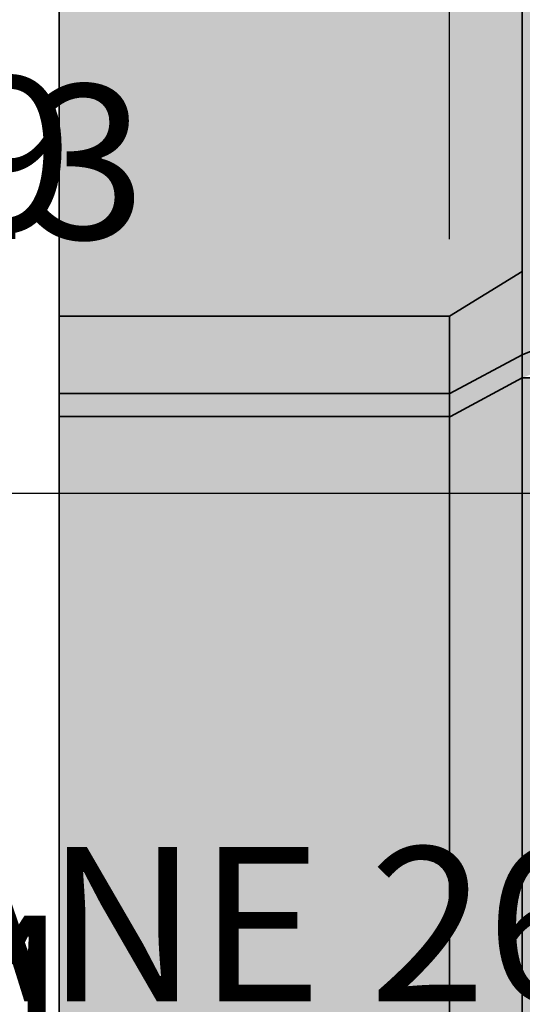
# Model space of a CAD drawing. Units: millimetres. Extents: x 130 to 1021, y 147 to 699.
# Tile 4 of 40: x 302 to 367, y 313 to 440. Entities that reach past the tile are written whole.
import ezdxf

# ---------------------------------------------------------------- set-up
doc = ezdxf.new("R2010")
doc.units = ezdxf.units.MM
doc.header["$MEASUREMENT"] = 0
for name, color, linetype, lineweight in [('A-ANNO-DIMS', 2, 'Continuous', 18), ('A-ELEV', 7, 'Continuous', 35), ('A-ELEV-PATT', 9, 'Continuous', 13)]:
    doc.layers.add(name, color=color, linetype=linetype, lineweight=lineweight)
doc.styles.get("Standard").update_dxf_attribs({"font": 'arial.ttf'})
doc.dimstyles.get("Standard").update_dxf_attribs({"dimtxt": 20, "dimasz": 10, "dimexe": 10, "dimexo": 10, "dimgap": 5, "dimtad": 0, "dimtih": 1, "dimtoh": 1, "dimdec": 0, "dimzin": 0, "dimdsep": 46, "dimtxsty": 'Standard', "dimcen": 5, "dimadec": 0, "dimazin": 0, "dimtfac": 1, "dimtdec": 0, "dimtofl": 0, "dimtmove": 0, "dimatfit": 3, "dimfxl": 1, "dimtolj": 1, "dimtzin": 0, "dimarcsym": 0})

# ---------------------------------------------------------------- blocks, each defined once
blk = doc.blocks.new('*D9')
at = {"layer": 'A-ANNO-DIMS', "color": 0, "lineweight": -2, "transparency": 16777216}
for p, q in [((467.37, 323.13), (457.37, 323.13)), ((467.37, 313.13), (467.37, 323.13)), ((473.55, 303.13), (477.38, 303.13)), ((473.57, 277.58), (477.4, 277.58)), ((467.41, 267.57), (467.42, 257.57))]:
    blk.add_line(p, q, dxfattribs=at)
at = {"layer": 'A-ANNO-DIMS', "color": 0, "transparency": 16777216}
for points in [[(469.04, 313.13), (465.71, 313.13), (467.38, 303.13)], [(469.08, 267.57), (465.75, 267.57), (467.4, 277.57)]]:
    blk.add_solid(points, dxfattribs=at)
at = {"layer": 'Defpoints', "color": 0, "transparency": 16777216}
for p in [(463.55, 303.12), (467.38, 303.13), (463.57, 277.57)]:
    blk.add_point(p, dxfattribs=at)
at = {"layer": 'A-ANNO-DIMS', "color": 0, "transparency": 16777216, "insert": (284.19, 323.13), "char_height": 20, "attachment_point": 5}
blk.add_mtext('\\A1;SIDELIGHT PANE 26 TYP.', dxfattribs=at)
blk = doc.blocks.new('*D11')
at = {"layer": 'A-ANNO-DIMS', "color": 0, "lineweight": -2, "transparency": 16777216}
for p, q in [((737.37, 648.7), (737.37, 149.74)), ((299.37, 566.95), (299.37, 149.74)), ((309.37, 159.74), (490.86, 159.74)), ((727.37, 159.74), (545.89, 159.74))]:
    blk.add_line(p, q, dxfattribs=at)
at = {"layer": 'A-ANNO-DIMS', "color": 0, "transparency": 16777216}
for points in [[(309.37, 161.41), (309.37, 158.07), (299.37, 159.74)], [(727.37, 161.41), (727.37, 158.07), (737.37, 159.74)]]:
    blk.add_solid(points, dxfattribs=at)
at = {"layer": 'Defpoints', "color": 0, "transparency": 16777216}
for p in [(737.37, 658.7), (299.37, 576.95), (737.37, 159.74)]:
    blk.add_point(p, dxfattribs=at)
at = {"layer": 'A-ANNO-DIMS', "color": 0, "transparency": 16777216, "insert": (518.37, 159.74), "char_height": 20, "attachment_point": 5}
blk.add_mtext('\\A1;438', dxfattribs=at)
blk = doc.blocks.new('*D12')
at = {"layer": 'A-ANNO-DIMS', "color": 0, "lineweight": -2, "transparency": 16777216}
for p, q in [((477.37, 661.95), (265.07, 661.95)), ((275.07, 651.95), (275.07, 438.2)), ((275.07, 194.04), (275.07, 407.78)), ((357.16, 184.04), (265.07, 184.04))]:
    blk.add_line(p, q, dxfattribs=at)
at = {"layer": 'A-ANNO-DIMS', "color": 0, "transparency": 16777216}
for points in [[(273.41, 651.95), (276.74, 651.95), (275.07, 661.95)], [(273.41, 194.04), (276.74, 194.04), (275.07, 184.04)]]:
    blk.add_solid(points, dxfattribs=at)
at = {"layer": 'Defpoints', "color": 0, "transparency": 16777216}
for p in [(275.07, 661.95), (487.37, 661.95), (367.16, 184.04)]:
    blk.add_point(p, dxfattribs=at)
at = {"layer": 'A-ANNO-DIMS', "color": 0, "transparency": 16777216, "insert": (275.07, 422.99), "char_height": 20, "attachment_point": 5}
blk.add_mtext('\\A1;477.9', dxfattribs=at)
blk = doc.blocks.new('*D15')
at = {"layer": 'A-ANNO-DIMS', "color": 0, "lineweight": -2, "transparency": 16777216}
for p, q in [((327.37, 579.88), (327.37, 696.25)), ((357.94, 411.95), (357.94, 696.25)), ((337.37, 686.25), (347.94, 686.25)), ((357.94, 686.25), (367.94, 686.25))]:
    blk.add_line(p, q, dxfattribs=at)
at = {"layer": 'A-ANNO-DIMS', "color": 0, "transparency": 16777216}
for points in [[(337.37, 687.91), (337.37, 684.58), (327.37, 686.25)], [(347.94, 687.91), (347.94, 684.58), (357.94, 686.25)]]:
    blk.add_solid(points, dxfattribs=at)
at = {"layer": 'Defpoints', "color": 0, "transparency": 16777216}
for p in [(357.94, 686.25), (327.37, 569.88), (357.94, 401.95)]:
    blk.add_point(p, dxfattribs=at)
at = {"layer": 'A-ANNO-DIMS', "color": 0, "transparency": 16777216, "insert": (406.68, 686.25), "char_height": 20, "attachment_point": 5}
blk.add_mtext('\\A1;30.57', dxfattribs=at)
blk = doc.blocks.new('*D16')
at = {"layer": 'A-ANNO-DIMS', "color": 0, "lineweight": -2, "transparency": 16777216}
for p, q in [((357.94, 411.95), (357.94, 696.25)), ((363.92, 579.88), (363.92, 696.25)), ((347.94, 686.25), (337.94, 686.25)), ((373.92, 686.25), (383.92, 686.25))]:
    blk.add_line(p, q, dxfattribs=at)
at = {"layer": 'A-ANNO-DIMS', "color": 0, "transparency": 16777216}
for points in [[(347.94, 687.91), (347.94, 684.58), (357.94, 686.25)], [(373.92, 687.91), (373.92, 684.58), (363.92, 686.25)]]:
    blk.add_solid(points, dxfattribs=at)
at = {"layer": 'Defpoints', "color": 0, "transparency": 16777216}
for p in [(363.92, 686.25), (363.92, 569.88), (357.94, 401.95)]:
    blk.add_point(p, dxfattribs=at)
at = {"layer": 'A-ANNO-DIMS', "color": 0, "transparency": 16777216, "insert": (420.74, 686.25), "char_height": 20, "attachment_point": 5}
blk.add_mtext('\\A1;5.981', dxfattribs=at)
blk = doc.blocks.new('*D18')
at = {"layer": 'A-ANNO-DIMS', "color": 0, "lineweight": -2, "transparency": 16777216}
for p, q in [((375.85, 490.22), (375.85, 696.25)), ((382.37, 388.95), (382.37, 696.25)), ((365.85, 686.25), (355.85, 686.25)), ((392.37, 686.25), (402.37, 686.25))]:
    blk.add_line(p, q, dxfattribs=at)
at = {"layer": 'A-ANNO-DIMS', "color": 0, "transparency": 16777216}
for points in [[(365.85, 687.91), (365.85, 684.58), (375.85, 686.25)], [(392.37, 687.91), (392.37, 684.58), (382.37, 686.25)]]:
    blk.add_solid(points, dxfattribs=at)
at = {"layer": 'Defpoints', "color": 0, "transparency": 16777216}
for p in [(382.37, 686.25), (375.85, 480.22), (382.37, 378.95)]:
    blk.add_point(p, dxfattribs=at)
at = {"layer": 'A-ANNO-DIMS', "color": 0, "transparency": 16777216, "insert": (441.13, 686.25), "char_height": 20, "attachment_point": 5}
blk.add_mtext('\\A1;6.524', dxfattribs=at)
blk = doc.blocks.new('*D38')
at = {"layer": 'A-ANNO-DIMS', "color": 0, "lineweight": -2, "transparency": 16777216}
for p, q in [((297.37, 388.95), (265.07, 388.95)), ((275.07, 378.95), (275.07, 346.66)), ((275.07, 283.95), (275.07, 316.24)), ((297.37, 273.95), (265.07, 273.95))]:
    blk.add_line(p, q, dxfattribs=at)
at = {"layer": 'A-ANNO-DIMS', "color": 0, "transparency": 16777216}
for points in [[(273.41, 378.95), (276.74, 378.95), (275.07, 388.95)], [(273.41, 283.95), (276.74, 283.95), (275.07, 273.95)]]:
    blk.add_solid(points, dxfattribs=at)
at = {"layer": 'Defpoints', "color": 0, "transparency": 16777216}
for p in [(275.07, 388.95), (307.37, 388.95), (307.37, 273.95)]:
    blk.add_point(p, dxfattribs=at)
at = {"layer": 'A-ANNO-DIMS', "color": 0, "transparency": 16777216, "insert": (275.07, 331.45), "char_height": 20, "attachment_point": 5}
blk.add_mtext('\\A1;115', dxfattribs=at)
blk = doc.blocks.new('*D39')
at = {"layer": 'A-ANNO-DIMS', "color": 0, "lineweight": -2, "transparency": 16777216}
for p, q in [((275.07, 411.95), (275.07, 421.95)), ((275.07, 421.95), (285.07, 421.95)), ((297.37, 401.95), (265.07, 401.95)), ((297.37, 388.95), (265.07, 388.95)), ((275.07, 378.95), (275.07, 368.95))]:
    blk.add_line(p, q, dxfattribs=at)
at = {"layer": 'A-ANNO-DIMS', "color": 0, "transparency": 16777216}
for points in [[(273.41, 411.95), (276.74, 411.95), (275.07, 401.95)], [(273.41, 378.95), (276.74, 378.95), (275.07, 388.95)]]:
    blk.add_solid(points, dxfattribs=at)
at = {"layer": 'Defpoints', "color": 0, "transparency": 16777216}
for p in [(275.07, 401.95), (307.37, 401.95), (307.37, 388.95)]:
    blk.add_point(p, dxfattribs=at)
at = {"layer": 'A-ANNO-DIMS', "color": 0, "transparency": 16777216, "insert": (303.46, 421.95), "char_height": 20, "attachment_point": 5}
blk.add_mtext('\\A1;13', dxfattribs=at)
blk = doc.blocks.new('*D40')
at = {"layer": 'A-ANNO-DIMS', "color": 0, "lineweight": -2, "transparency": 16777216}
for p, q in [((292.37, 463.95), (265.07, 463.95)), ((275.07, 453.95), (275.07, 448.16)), ((275.07, 411.95), (275.07, 417.74)), ((297.37, 401.95), (265.07, 401.95))]:
    blk.add_line(p, q, dxfattribs=at)
at = {"layer": 'A-ANNO-DIMS', "color": 0, "transparency": 16777216}
for points in [[(273.41, 453.95), (276.74, 453.95), (275.07, 463.95)], [(273.41, 411.95), (276.74, 411.95), (275.07, 401.95)]]:
    blk.add_solid(points, dxfattribs=at)
at = {"layer": 'Defpoints', "color": 0, "transparency": 16777216}
for p in [(275.07, 463.95), (302.37, 463.95), (307.37, 401.95)]:
    blk.add_point(p, dxfattribs=at)
at = {"layer": 'A-ANNO-DIMS', "color": 0, "transparency": 16777216, "insert": (275.07, 432.95), "char_height": 20, "attachment_point": 5}
blk.add_mtext('\\A1;62', dxfattribs=at)
blk = doc.blocks.new('*D60')
at = {"layer": 'A-ANNO-DIMS', "color": 0, "lineweight": -2, "transparency": 16777216}
for p, q in [((372.37, 378.95), (265.07, 378.95)), ((275.07, 368.95), (275.07, 329.46)), ((275.07, 259.55), (275.07, 299.04)), ((372.37, 249.55), (265.07, 249.55))]:
    blk.add_line(p, q, dxfattribs=at)
at = {"layer": 'A-ANNO-DIMS', "color": 0, "transparency": 16777216}
for points in [[(273.41, 368.95), (276.74, 368.95), (275.07, 378.95)], [(273.41, 259.55), (276.74, 259.55), (275.07, 249.55)]]:
    blk.add_solid(points, dxfattribs=at)
at = {"layer": 'Defpoints', "color": 0, "transparency": 16777216}
for p in [(275.07, 378.95), (382.37, 378.95), (382.37, 249.55)]:
    blk.add_point(p, dxfattribs=at)
at = {"layer": 'A-ANNO-DIMS', "color": 0, "transparency": 16777216, "insert": (275.07, 314.25), "char_height": 20, "attachment_point": 5}
blk.add_mtext('\\A1;129.4', dxfattribs=at)
blk = doc.blocks.new('*D64')
at = {"layer": 'A-ANNO-DIMS', "color": 0, "lineweight": -2, "transparency": 16777216}
for p, q in [((502.05, 450.93), (502.05, 460.93)), ((497.05, 455.93), (507.05, 455.93)), ((363.96, 263.06), (409.92, 327.25)), ((353.96, 263.06), (363.96, 263.06))]:
    blk.add_line(p, q, dxfattribs=at)
at = {"layer": 'A-ANNO-DIMS', "color": 0, "transparency": 16777216}
blk.add_solid([(408.57, 328.22), (411.28, 326.28), (415.74, 335.39)], dxfattribs=at)
at = {"layer": 'Defpoints', "color": 0, "transparency": 16777216}
for p in [(502.05, 455.93), (415.74, 335.39)]:
    blk.add_point(p, dxfattribs=at)
at = {"layer": 'A-ANNO-DIMS', "color": 0, "transparency": 16777216, "insert": (297.8, 263.06), "char_height": 20, "attachment_point": 5}
blk.add_mtext('\\A1;R148.25', dxfattribs=at)
blk = doc.blocks.new('*D66')
at = {"layer": 'A-ANNO-DIMS', "color": 0, "lineweight": -2, "transparency": 16777216}
for p, q in [((341.58, 557.19), (351.58, 557.19)), ((351.58, 557.19), (376.95, 478.14)), ((427.37, 315.98), (427.37, 325.98)), ((422.37, 320.98), (432.37, 320.98))]:
    blk.add_line(p, q, dxfattribs=at)
at = {"layer": 'A-ANNO-DIMS', "color": 0, "transparency": 16777216}
blk.add_solid([(378.53, 478.64), (375.36, 477.63), (380, 468.61)], dxfattribs=at)
at = {"layer": 'Defpoints', "color": 0, "transparency": 16777216}
for p in [(380, 468.61), (427.37, 320.98)]:
    blk.add_point(p, dxfattribs=at)
at = {"layer": 'A-ANNO-DIMS', "color": 0, "transparency": 16777216, "insert": (263.53, 557.19), "char_height": 20, "attachment_point": 5}
blk.add_mtext('\\A1;4X R155.05', dxfattribs=at)
blk = doc.blocks.new('*D68')
at = {"layer": 'A-ANNO-DIMS', "color": 0, "lineweight": -2, "transparency": 16777216}
for p, q in [((361.84, 579.76), (371.84, 579.76)), ((371.84, 579.76), (392.17, 506.69)), ((433.19, 354.23), (433.19, 364.23)), ((428.19, 359.23), (438.19, 359.23))]:
    blk.add_line(p, q, dxfattribs=at)
at = {"layer": 'A-ANNO-DIMS', "color": 0, "transparency": 16777216}
blk.add_solid([(393.77, 507.14), (390.56, 506.25), (394.85, 497.06)], dxfattribs=at)
at = {"layer": 'Defpoints', "color": 0, "transparency": 16777216}
for p in [(394.85, 497.06), (433.19, 359.23)]:
    blk.add_point(p, dxfattribs=at)
at = {"layer": 'A-ANNO-DIMS', "color": 0, "transparency": 16777216, "insert": (305.76, 579.76), "char_height": 20, "attachment_point": 5}
blk.add_mtext('\\A1;R143.06', dxfattribs=at)
blk = doc.blocks.new('*D70')
at = {"layer": 'A-ANNO-DIMS', "color": 0, "lineweight": -2, "transparency": 16777216}
for p, q in [((370.14, 588.4), (380.14, 588.4)), ((380.14, 588.4), (397.47, 517.01)), ((432.65, 367.11), (432.65, 377.11)), ((427.65, 372.11), (437.65, 372.11))]:
    blk.add_line(p, q, dxfattribs=at)
at = {"layer": 'A-ANNO-DIMS', "color": 0, "transparency": 16777216}
blk.add_solid([(399.09, 517.4), (395.85, 516.62), (399.83, 507.29)], dxfattribs=at)
at = {"layer": 'Defpoints', "color": 0, "transparency": 16777216}
for p in [(399.83, 507.29), (432.65, 372.11)]:
    blk.add_point(p, dxfattribs=at)
at = {"layer": 'A-ANNO-DIMS', "color": 0, "transparency": 16777216, "insert": (323.76, 588.4), "char_height": 20, "attachment_point": 5}
blk.add_mtext('\\A1;R139.1', dxfattribs=at)
blk = doc.blocks.new('*D73')
at = {"layer": 'A-ANNO-DIMS', "color": 0, "lineweight": -2, "transparency": 16777216}
for p, q in [((402.68, 571.45), (412.68, 571.45)), ((412.68, 571.45), (419.05, 502.17)), ((432.11, 355.14), (432.11, 365.14)), ((427.11, 360.14), (437.11, 360.14))]:
    blk.add_line(p, q, dxfattribs=at)
at = {"layer": 'A-ANNO-DIMS', "color": 0, "transparency": 16777216}
blk.add_solid([(420.71, 502.32), (417.39, 502.01), (419.97, 492.21)], dxfattribs=at)
at = {"layer": 'Defpoints', "color": 0, "transparency": 16777216}
for p in [(419.97, 492.21), (432.11, 360.14)]:
    blk.add_point(p, dxfattribs=at)
at = {"layer": 'A-ANNO-DIMS', "color": 0, "transparency": 16777216, "insert": (346.7, 571.45), "char_height": 20, "attachment_point": 5}
blk.add_mtext('\\A1;R132.62', dxfattribs=at)

msp = doc.modelspace()

# ---------------------------------------------------------------- hatches: boundary and pattern name
at = {"layer": 'A-ELEV-PATT'}
h = msp.add_hatch(color=256, dxfattribs=at)
h.dxf.hatch_style = 1
h.paths.add_polyline_path([(737.3738, 658.6988, 0.01359606), (632.4019, 661.9473), (607.3738, 661.9473), (487.3738, 661.9473), (487.3738, 649.9473), (607.3738, 649.9473), (632.3794, 649.9473, -0.01368411), (737.3738, 646.6784)])
h.paths.add_polyline_path([(732.3738, 643.9599, 0.01305286), (632.3738, 646.9473), (607.3738, 646.9473), (487.3738, 646.9473), (487.3738, 596.9473), (632.3738, 596.9473, -0.01305286), (732.3738, 593.9599)])
h.paths.add_polyline_path([(737.3738, 593.6732, 0.01370629), (632.3738, 596.9473), (487.3738, 596.9473), (487.3738, 586.9473), (632.355, 586.9473, -0.01378075), (737.3738, 583.6559)])
h.paths.add_polyline_path([(447.3738, 646.9473), (307.3738, 646.9473), (302.3738, 646.9473), (302.3738, 634.9473), (447.3738, 634.9473)])
h.paths.add_polyline_path([(447.3738, 631.9473), (307.3738, 631.9473), (307.3738, 586.9473), (447.3738, 586.9473)])
h.paths.add_polyline_path([(447.3738, 586.9473), (307.3738, 586.9473), (302.3738, 586.9473), (302.3738, 576.9473), (447.3738, 576.9473)])
h.paths.add_polyline_path([(447.3738, 573.9473), (367.3738, 573.9473), (367.3738, 539.9473), (447.3738, 539.9473)])
h.paths.add_polyline_path([(447.3738, 537.9473), (367.3738, 537.9473), (367.3738, 507.9473), (400.392, 507.4253, -0.00172798), (401.3281, 507.6451, -0.52200255), (425.6117, 511.0391, -0.03918489), (447.3738, 510.4359), (447.3738, 510.7883)])
h.paths.add_polyline_path([(394.7238, 505.9473), (367.3738, 505.9473), (367.3738, 476.9473, -0.0146512), (375.8501, 480.2159), (376.1506, 499.2266, -0.03554194)])
h.paths.add_polyline_path([(632.3738, 583.9473), (552.3738, 583.9473), (552.3738, 550.9473), (632.3738, 550.9473)])
h.paths.add_polyline_path([(632.3738, 548.9473), (552.3738, 548.9473), (552.3738, 515.9473), (632.3738, 515.9473)])
h.paths.add_polyline_path([(632.3738, 513.9473), (552.3738, 513.9473), (552.3738, 476.9473), (632.3738, 476.9473)])
h.paths.add_polyline_path([(737.3738, 473.6903, 0.01363261), (632.3926, 476.9473), (552.3738, 476.9473), (487.3738, 476.9473), (487.3738, 466.9473), (632.3738, 466.9473, -0.01370629), (737.3738, 463.6732)])
h.paths.add_polyline_path([(732.3738, 460.9552, 0.01307409), (632.3681, 463.9473), (487.3738, 463.9473), (487.3738, 407.735, -0.00322862), (489.3544, 406.9473), (632.3926, 406.9473, -0.01298259), (732.3738, 403.9755)])
h.paths.add_polyline_path([(487.3738, 463.9473, 0.20132998), (367.3738, 463.9473), (367.3738, 407.735, -0.18820307), (487.3738, 407.735)])
h.paths.add_polyline_path([(367.3738, 476.9473), (367.3738, 466.9473, -0.20133085), (487.3738, 466.9473), (487.3738, 476.9473, 0.20132998)])
h.paths.add_polyline_path([(367.3738, 463.9473), (307.3738, 463.9473), (307.3738, 401.9473), (357.9413, 401.9473), (367.3738, 407.735)])
h.paths.add_polyline_path([(367.3738, 476.9473), (302.3738, 476.9473), (302.3738, 466.9473), (367.3738, 466.9473)])
h.paths.add_polyline_path([(632.8184, 366.9453), (552.3738, 366.9453), (552.3738, 393.9473), (632.8184, 393.9473)])
h.paths.add_polyline_path([(632.8184, 357.2114), (632.8184, 363.9453), (552.3738, 363.9453), (552.3738, 357.2114), (552.3738, 336.9453), (632.8184, 336.9453)])
h.paths.add_polyline_path([(632.8184, 333.9453), (552.3738, 333.9453), (552.3738, 306.9453), (632.8184, 306.9453)])
h.paths.add_polyline_path([(632.8184, 303.9453), (552.3738, 303.9453), (552.3738, 273.9473), (632.355, 273.9473, 0.00006077), (632.8184, 273.9491)])
h.paths.add_polyline_path([(737.3738, 403.6903, 0.01363261), (632.3926, 406.9473), (489.3544, 406.9473, 0.19154808), (367.3738, 407.735), (367.3738, 396.9473, -0.20133085), (487.3738, 396.9473), (632.3738, 396.9473, -0.01370629), (737.3738, 393.6732)])
h.paths.add_polyline_path([(357.9413, 401.9473), (307.3738, 401.9473), (307.3738, 391.9473), (357.9413, 391.9473)])
h.paths.add_polyline_path([(357.9413, 357.2114), (357.9413, 388.9473), (307.3738, 388.9473), (307.3738, 357.2114), (307.3738, 273.9473), (357.9413, 273.9473)])
h.paths.add_polyline_path([(732.3738, 263.93, -0.0130317), (632.3794, 260.9473), (466.7667, 260.9473), (466.7667, 240.9473), (469.8406, 236.978), (469.8406, 221.978), (472.9145, 218.0087), (472.9145, 213.9473), (607.3738, 213.9473), (732.3738, 213.9473)])
h.paths.add_polyline_path([(732.3738, 290.889), (722.479, 290.889), (722.479, 301.889), (732.3738, 301.889), (732.3738, 305.889), (722.479, 305.889), (722.479, 316.889), (732.3738, 316.889), (732.3738, 320.889), (722.479, 320.889), (722.479, 331.889), (732.3738, 331.889), (732.3738, 335.889), (722.479, 335.889), (722.479, 346.889), (732.3738, 346.889), (732.3738, 350.889), (722.479, 350.889), (722.479, 361.889), (732.3738, 361.889), (732.3738, 365.889), (722.479, 365.889), (722.479, 376.889), (732.3738, 376.889), (732.3738, 380.889), (722.479, 380.889), (722.479, 391.4848, 0.00052326), (718.479, 391.6843), (718.479, 380.889), (707.479, 380.889), (707.479, 392.1896, 0.00052307), (703.479, 392.3576), (703.479, 380.889), (692.479, 380.889), (692.479, 392.7765, 0.00052292), (688.479, 392.9131), (688.479, 380.889), (677.479, 380.889), (677.479, 393.2456, 0.00052279), (673.479, 393.3508), (673.479, 380.889), (662.479, 380.889), (662.479, 393.597, 0.0005227), (658.479, 393.6709), (658.479, 380.889), (647.479, 380.889), (647.479, 393.8308, 0.00052264), (643.479, 393.8732), (643.479, 380.889), (632.8184, 380.889), (632.8184, 376.889), (643.479, 376.889), (643.479, 365.889), (632.8184, 365.889), (632.8184, 361.889), (643.479, 361.889), (643.479, 350.889), (632.8184, 350.889), (632.8184, 346.889), (643.479, 346.889), (643.479, 335.889), (632.8184, 335.889), (632.8184, 331.889), (643.479, 331.889), (643.479, 320.889), (632.8184, 320.889), (632.8184, 316.889), (643.479, 316.889), (643.479, 305.889), (632.8184, 305.889), (632.8184, 301.889), (643.479, 301.889), (643.479, 290.889), (632.8184, 290.889), (632.8184, 286.889), (643.479, 286.889), (643.479, 274.0217, 0.00052456), (647.479, 274.0643), (647.479, 286.889), (658.479, 286.889), (658.479, 274.2248, 0.00052462), (662.479, 274.2989), (662.479, 286.889), (673.479, 286.889), (673.479, 274.546, 0.00052471), (677.479, 274.6516), (677.479, 286.889), (688.479, 286.889), (688.479, 274.9853, 0.00052484), (692.479, 275.1224), (692.479, 286.889), (703.479, 286.889), (703.479, 275.5429, 0.000525), (707.479, 275.7115), (707.479, 286.889), (718.479, 286.889), (718.479, 276.2187, 0.00052519), (722.479, 276.4189), (722.479, 286.889), (732.3738, 286.889)])
h.paths.add_polyline_path([(718.479, 290.889), (707.479, 290.889), (707.479, 301.889), (718.479, 301.889)], flags=16)
h.paths.add_polyline_path([(703.479, 290.889), (692.479, 290.889), (692.479, 301.889), (703.479, 301.889)], flags=16)
h.paths.add_polyline_path([(718.479, 305.889), (707.479, 305.889), (707.479, 316.889), (718.479, 316.889)], flags=16)
h.paths.add_polyline_path([(703.479, 305.889), (692.479, 305.889), (692.479, 316.889), (703.479, 316.889)], flags=16)
h.paths.add_polyline_path([(688.479, 290.889), (677.479, 290.889), (677.479, 301.889), (688.479, 301.889)], flags=16)
h.paths.add_polyline_path([(718.479, 320.889), (707.479, 320.889), (707.479, 331.889), (718.479, 331.889)], flags=16)
h.paths.add_polyline_path([(688.479, 305.889), (677.479, 305.889), (677.479, 316.889), (688.479, 316.889)], flags=16)
h.paths.add_polyline_path([(703.479, 320.889), (692.479, 320.889), (692.479, 331.889), (703.479, 331.889)], flags=16)
h.paths.add_polyline_path([(688.479, 320.889), (677.479, 320.889), (677.479, 331.889), (688.479, 331.889)], flags=16)
h.paths.add_polyline_path([(673.479, 290.889), (662.479, 290.889), (662.479, 301.889), (673.479, 301.889)], flags=16)
h.paths.add_polyline_path([(718.479, 335.889), (707.479, 335.889), (707.479, 346.889), (718.479, 346.889)], flags=16)
h.paths.add_polyline_path([(673.479, 305.889), (662.479, 305.889), (662.479, 316.889), (673.479, 316.889)], flags=16)
h.paths.add_polyline_path([(703.479, 335.889), (692.479, 335.889), (692.479, 346.889), (703.479, 346.889)], flags=16)
h.paths.add_polyline_path([(673.479, 320.889), (662.479, 320.889), (662.479, 331.889), (673.479, 331.889)], flags=16)
h.paths.add_polyline_path([(688.479, 335.889), (677.479, 335.889), (677.479, 346.889), (688.479, 346.889)], flags=16)
h.paths.add_polyline_path([(658.479, 290.889), (647.479, 290.889), (647.479, 301.889), (658.479, 301.889)], flags=16)
h.paths.add_polyline_path([(718.479, 350.889), (707.479, 350.889), (707.479, 361.889), (718.479, 361.889)], flags=16)
h.paths.add_polyline_path([(658.479, 305.889), (647.479, 305.889), (647.479, 316.889), (658.479, 316.889)], flags=16)
h.paths.add_polyline_path([(703.479, 350.889), (692.479, 350.889), (692.479, 361.889), (703.479, 361.889)], flags=16)
h.paths.add_polyline_path([(673.479, 335.889), (662.479, 335.889), (662.479, 346.889), (673.479, 346.889)], flags=16)
h.paths.add_polyline_path([(658.479, 320.889), (647.479, 320.889), (647.479, 331.889), (658.479, 331.889)], flags=16)
h.paths.add_polyline_path([(688.479, 350.889), (677.479, 350.889), (677.479, 361.889), (688.479, 361.889)], flags=16)
h.paths.add_polyline_path([(718.479, 365.889), (707.479, 365.889), (707.479, 376.889), (718.479, 376.889)], flags=16)
h.paths.add_polyline_path([(658.479, 335.889), (647.479, 335.889), (647.479, 346.889), (658.479, 346.889)], flags=16)
h.paths.add_polyline_path([(673.479, 350.889), (662.479, 350.889), (662.479, 361.889), (673.479, 361.889)], flags=16)
h.paths.add_polyline_path([(703.479, 365.889), (692.479, 365.889), (692.479, 376.889), (703.479, 376.889)], flags=16)
h.paths.add_polyline_path([(688.479, 365.889), (677.479, 365.889), (677.479, 376.889), (688.479, 376.889)], flags=16)
h.paths.add_polyline_path([(658.479, 350.889), (647.479, 350.889), (647.479, 361.889), (658.479, 361.889)], flags=16)
h.paths.add_polyline_path([(673.479, 365.889), (662.479, 365.889), (662.479, 376.889), (673.479, 376.889)], flags=16)
h.paths.add_polyline_path([(658.479, 365.889), (647.479, 365.889), (647.479, 376.889), (658.479, 376.889)], flags=16)
h.paths.add_polyline_path([(732.3738, 503.9786), (722.3392, 503.9786), (722.3392, 514.9786), (732.3738, 514.9786), (732.3738, 518.9786), (722.3392, 518.9786), (722.3392, 529.9786), (732.3738, 529.9786), (732.3738, 533.9786), (722.3392, 533.9786), (722.3392, 544.9786), (732.3738, 544.9786), (732.3738, 546.9473), (732.3738, 548.9786), (722.3392, 548.9786), (722.3392, 559.9786), (732.3738, 559.9786), (732.3738, 563.9786), (722.3392, 563.9786), (722.3392, 574.9786), (732.3738, 574.9786), (732.3738, 578.9786), (722.3392, 578.9786), (722.3392, 581.4789, 0.00052601), (718.3392, 581.6791), (718.3392, 578.9786), (707.3392, 578.9786), (707.3392, 582.1863, 0.00052582), (703.3392, 582.355), (703.3392, 578.9786), (692.3392, 578.9786), (692.3392, 582.7752, 0.00052566), (688.3392, 582.9123), (688.3392, 578.9786), (677.3392, 578.9786), (677.3392, 583.2457, 0.00052554), (673.3392, 583.3512), (673.3392, 578.9786), (662.3392, 578.9786), (662.3392, 583.5978, 0.00052545), (658.3392, 583.6718), (658.3392, 578.9786), (647.3392, 578.9786), (647.3392, 583.8317, 0.00052539), (643.3392, 583.8741), (643.3392, 578.9786), (632.3738, 578.9786), (632.3738, 574.9786), (643.3392, 574.9786), (643.3392, 563.9786), (632.3738, 563.9786), (632.3738, 559.9786), (643.3392, 559.9786), (643.3392, 548.9786), (632.3738, 548.9786), (632.3738, 544.9786), (643.3392, 544.9786), (643.3392, 533.9786), (632.3738, 533.9786), (632.3738, 529.9786), (643.3392, 529.9786), (643.3392, 518.9786), (632.3738, 518.9786), (632.3738, 515.9473), (632.3738, 514.9786), (643.3392, 514.9786), (643.3392, 503.9786), (632.3738, 503.9786), (632.3738, 499.9786), (643.3392, 499.9786), (643.3392, 488.9786), (632.3738, 488.9786), (632.3738, 484.9786), (643.3392, 484.9786), (643.3392, 476.8751, -0.00051911), (647.3392, 476.8332), (647.3392, 484.9786), (658.3392, 484.9786), (658.3392, 476.6752, -0.00051917), (662.3392, 476.6022), (662.3392, 484.9786), (673.3392, 484.9786), (673.3392, 476.3585, -0.00051926), (677.3392, 476.2543), (677.3392, 484.9786), (688.3392, 484.9786), (688.3392, 475.9248, -0.00051938), (692.3392, 475.7894), (692.3392, 484.9786), (703.3392, 484.9786), (703.3392, 475.3741, -0.00051953), (707.3392, 475.2075), (707.3392, 484.9786), (718.3392, 484.9786), (718.3392, 474.7064, -0.00051972), (722.3392, 474.5086), (722.3392, 484.9786), (732.3738, 484.9786), (732.3738, 488.9786), (722.3392, 488.9786), (722.3392, 499.9786), (732.3738, 499.9786)])
h.paths.add_polyline_path([(718.3392, 503.9786), (707.3392, 503.9786), (707.3392, 514.9786), (718.3392, 514.9786)], flags=16)
h.paths.add_polyline_path([(718.3392, 499.9786), (718.3392, 488.9786), (707.3392, 488.9786), (707.3392, 499.9786)], flags=16)
h.paths.add_polyline_path([(718.3392, 518.9786), (707.3392, 518.9786), (707.3392, 529.9786), (718.3392, 529.9786)], flags=16)
h.paths.add_polyline_path([(703.3392, 503.9786), (692.3392, 503.9786), (692.3392, 514.9786), (703.3392, 514.9786)], flags=16)
h.paths.add_polyline_path([(703.3392, 499.9786), (703.3392, 488.9786), (692.3392, 488.9786), (692.3392, 499.9786)], flags=16)
h.paths.add_polyline_path([(703.3392, 518.9786), (692.3392, 518.9786), (692.3392, 529.9786), (703.3392, 529.9786)], flags=16)
h.paths.add_polyline_path([(718.3392, 533.9786), (707.3392, 533.9786), (707.3392, 544.9786), (718.3392, 544.9786)], flags=16)
h.paths.add_polyline_path([(688.3392, 503.9786), (677.3392, 503.9786), (677.3392, 514.9786), (688.3392, 514.9786)], flags=16)
h.paths.add_polyline_path([(688.3392, 499.9786), (688.3392, 488.9786), (677.3392, 488.9786), (677.3392, 499.9786)], flags=16)
h.paths.add_polyline_path([(703.3392, 533.9786), (692.3392, 533.9786), (692.3392, 544.9786), (703.3392, 544.9786)], flags=16)
h.paths.add_polyline_path([(688.3392, 518.9786), (677.3392, 518.9786), (677.3392, 529.9786), (688.3392, 529.9786)], flags=16)
h.paths.add_polyline_path([(688.3392, 533.9786), (677.3392, 533.9786), (677.3392, 544.9786), (688.3392, 544.9786)], flags=16)
h.paths.add_polyline_path([(718.3392, 548.9786), (707.3392, 548.9786), (707.3392, 559.9786), (718.3392, 559.9786)], flags=16)
h.paths.add_polyline_path([(673.3392, 503.9786), (662.3392, 503.9786), (662.3392, 514.9786), (673.3392, 514.9786)], flags=16)
h.paths.add_polyline_path([(673.3392, 499.9786), (673.3392, 488.9786), (662.3392, 488.9786), (662.3392, 499.9786)], flags=16)
h.paths.add_polyline_path([(703.3392, 548.9786), (692.3392, 548.9786), (692.3392, 559.9786), (703.3392, 559.9786)], flags=16)
h.paths.add_polyline_path([(673.3392, 518.9786), (662.3392, 518.9786), (662.3392, 529.9786), (673.3392, 529.9786)], flags=16)
h.paths.add_polyline_path([(688.3392, 548.9786), (677.3392, 548.9786), (677.3392, 559.9786), (688.3392, 559.9786)], flags=16)
h.paths.add_polyline_path([(673.3392, 533.9786), (662.3392, 533.9786), (662.3392, 544.9786), (673.3392, 544.9786)], flags=16)
h.paths.add_polyline_path([(718.3392, 563.9786), (707.3392, 563.9786), (707.3392, 574.9786), (718.3392, 574.9786)], flags=16)
h.paths.add_polyline_path([(658.3392, 503.9786), (647.3392, 503.9786), (647.3392, 514.9786), (658.3392, 514.9786)], flags=16)
h.paths.add_polyline_path([(658.3392, 499.9786), (658.3392, 488.9786), (647.3392, 488.9786), (647.3392, 499.9786)], flags=16)
h.paths.add_polyline_path([(703.3392, 563.9786), (692.3392, 563.9786), (692.3392, 574.9786), (703.3392, 574.9786)], flags=16)
h.paths.add_polyline_path([(658.3392, 518.9786), (647.3392, 518.9786), (647.3392, 529.9786), (658.3392, 529.9786)], flags=16)
h.paths.add_polyline_path([(673.3392, 548.9786), (662.3392, 548.9786), (662.3392, 559.9786), (673.3392, 559.9786)], flags=16)
h.paths.add_polyline_path([(688.3392, 563.9786), (677.3392, 563.9786), (677.3392, 574.9786), (688.3392, 574.9786)], flags=16)
h.paths.add_polyline_path([(658.3392, 533.9786), (647.3392, 533.9786), (647.3392, 544.9786), (658.3392, 544.9786)], flags=16)
h.paths.add_polyline_path([(673.3392, 563.9786), (662.3392, 563.9786), (662.3392, 574.9786), (673.3392, 574.9786)], flags=16)
h.paths.add_polyline_path([(658.3392, 548.9786), (647.3392, 548.9786), (647.3392, 559.9786), (658.3392, 559.9786)], flags=16)
h.paths.add_polyline_path([(658.3392, 563.9786), (647.3392, 563.9786), (647.3392, 574.9786), (658.3392, 574.9786)], flags=16)
h = msp.add_hatch(color=256, dxfattribs=at)
h.dxf.hatch_style = 1
h.paths.add_polyline_path([(447.3738, 576.9473), (302.3738, 576.9473), (302.3738, 573.9473), (447.3738, 573.9473)])
h.paths.add_polyline_path([(487.3738, 583.9473), (487.3738, 586.9473), (447.3738, 576.9473), (447.3738, 573.9473)])
h.paths.add_polyline_path([(632.355, 586.9473), (487.3738, 586.9473), (487.3738, 583.9473), (632.3738, 583.9473), (632.3738, 583.9472, -0.01380003), (737.3738, 580.6507), (737.3738, 583.6559, 0.01378075)])
h.paths.add_polyline_path([(367.3738, 466.9473), (302.3738, 466.9473), (302.3738, 463.9473), (367.3738, 463.9473)])
h.paths.add_polyline_path([(487.3738, 463.9473), (487.3738, 466.9473, 0.20133085), (367.3738, 466.9473), (367.3738, 463.9473, -0.20132998)])
h.paths.add_polyline_path([(632.3738, 466.9473), (487.3738, 466.9473), (487.3738, 463.9473), (632.3681, 463.9473, -0.01372855), (737.3738, 460.6681), (737.3738, 463.6732, 0.01370629)])
h.paths.add_polyline_path([(632.3738, 396.9473), (487.3738, 396.9473, 0.20133085), (367.3738, 396.9473), (367.3738, 393.9473, -0.20237172), (486.7667, 393.9473), (632.3681, 393.9473, -0.01372855), (737.3738, 390.6681), (737.3738, 393.6732, 0.01370629)])
h.paths.add_polyline_path([(357.9413, 391.9473), (307.3738, 391.9473), (307.3738, 388.9473), (357.9413, 388.9473)])
h.paths.add_polyline_path([(367.3738, 393.9473), (367.3738, 396.9473), (357.9413, 391.924), (357.9413, 388.9473), (358.058, 388.9473)])
h.paths.add_polyline_path([(737.3738, 264.2162), (737.3738, 267.2214, -0.01370629), (632.3738, 263.9473), (463.7667, 263.9473), (466.7667, 260.9473), (632.3794, 260.9473, 0.01368411)])
h.paths.add_polyline_path([(463.7667, 263.9473), (447.3738, 263.9473), (450.3738, 260.9473), (466.7667, 260.9473)])
h.paths.add_polyline_path([(447.3738, 263.9473), (432.3738, 263.9473), (432.3738, 260.9473), (450.3738, 260.9473)])
h.paths.add_polyline_path([(382.3738, 263.9473), (357.9413, 263.9473), (357.9413, 260.9473), (382.3738, 260.9473)])
h.paths.add_polyline_path([(357.9413, 263.9473), (307.3738, 263.9473), (307.3738, 260.9473), (357.9413, 260.9473)])
h = msp.add_hatch(color=256, dxfattribs=at)
h.dxf.hatch_style = 1
h.paths.add_polyline_path([(363.922, 569.884), (327.3738, 569.884), (327.3738, 557.9168), (363.922, 557.9168)])
h.paths.add_polyline_path([(547.7773, 577.3739), (502.3738, 577.3739), (502.3738, 566.2111), (547.7773, 566.2111)])
h.paths.add_polyline_path([(544.6354, 386.2639), (486.7667, 386.2639), (486.7667, 377.43), (544.6354, 377.43)])
h.paths.add_polyline_path([(496.0546, 377.43), (486.7667, 377.43), (486.7667, 370.4028)])
h.paths.add_polyline_path([(447.3738, 393.9473), (367.3738, 393.9473, 0.05004781), (382.3738, 368.424), (382.3738, 378.9473), (432.3738, 378.9473), (432.3738, 325.067, 0.02789446), (447.3738, 318.1243), (447.3738, 357.2114)])
h.paths.add_polyline_path([(463.5608, 388.6449), (450.8779, 388.6449), (450.8779, 363.0915), (463.5608, 363.0915)])
h.paths.add_polyline_path([(463.5608, 360.0915), (450.8779, 360.0915), (450.8779, 334.5915), (463.5608, 334.5915)])
h.paths.add_polyline_path([(463.5608, 331.5915), (450.8779, 331.5915), (450.8779, 316.785, 0.02245133), (463.5608, 312.7571)])
h = msp.add_hatch(color=256, dxfattribs=at)
h.dxf.hatch_style = 1
h.paths.add_polyline_path([(367.3738, 407.735), (357.9413, 401.9473), (357.9413, 391.9473), (357.985, 391.9473), (367.3738, 396.9473)])
h.paths.add_polyline_path([(367.3738, 393.9473), (357.9413, 388.8847), (357.9413, 357.2114), (357.9413, 273.9473), (367.3738, 273.9473), (367.3738, 357.2114)])
h = msp.add_hatch(color=256, dxfattribs=at)
h.dxf.hatch_style = 1
h.paths.add_polyline_path([(382.3738, 368.424, -0.05004781), (367.3738, 393.9473), (367.3738, 357.2114), (367.3738, 273.9473), (382.3738, 273.9473)])
h.paths.add_polyline_path([(432.3738, 273.9473), (447.3738, 273.9473), (447.3738, 318.1243, -0.02789446), (432.3738, 325.067)])
h.paths.add_polyline_path([(463.5608, 306.0915), (463.5608, 312.7571, -0.02245133), (450.8779, 316.785), (450.8779, 306.0915)])
h.paths.add_polyline_path([(450.8779, 303.0915), (450.8779, 277.5915), (463.5608, 277.5915), (463.5608, 303.0915)])

# ---------------------------------------------------------------- linework, layer by layer
at = {"layer": 'A-ELEV'}
for p, q in [((367.3738, 573.9473), (367.3738, 357.2114)), ((307.3738, 463.9473), (307.3738, 357.2114)), ((357.9413, 401.9473), (367.3738, 407.735)), ((357.9413, 401.9473), (307.3738, 401.9473)), ((357.9413, 401.9473), (357.9413, 357.2114)), ((357.985, 391.9473), (367.3738, 396.9473)), ((358.058, 388.9473), (367.3738, 393.9473)), ((632.3738, 393.9473), (367.3738, 393.9473)), ((357.985, 391.9473), (307.3738, 391.9473)), ((358.0549, 388.9473), (307.3738, 388.9473)), ((307.3738, 357.2114), (307.3738, 213.9473)), ((357.9413, 357.2114), (357.9413, 273.9473)), ((367.3738, 357.2114), (367.3738, 273.9473))]:
    msp.add_line(p, q, dxfattribs=at)
msp.add_arc((427.3738, 253.9788), 155.0484, 67.233534, 112.766466, dxfattribs=at)

# ---------------------------------------------------------------- dimensions: what is measured, and where the dimension line sits
at = {"layer": 'A-ANNO-DIMS'}
for base, p1, p2, override, picture, middle in [((357.9413, 686.2473), (327.3738, 569.884), (357.9413, 401.9473), {"dimdec": 2, "dimlfac": 1, "dimrnd": 0, "dimzin": 0, "dimdsep": 46, "dimlunit": 2}, '*D15', (406.6794, 686.2473)), ((363.922, 686.2473), (357.9413, 401.9473), (363.922, 569.884), {"dimdec": 3, "dimlfac": 1, "dimrnd": 0, "dimzin": 0, "dimdsep": 46, "dimlunit": 2}, '*D16', (420.7365, 686.2473)), ((382.3738, 686.2473), (375.8501, 480.2159), (382.3738, 378.9473), {"dimdec": 3, "dimlfac": 1, "dimrnd": 0, "dimzin": 0, "dimdsep": 46, "dimlunit": 2}, '*D18', (441.1323, 686.2473)), ((737.3738, 159.7395), (299.3738, 576.9473), (737.3738, 658.6988), {"dimdec": 0, "dimlfac": 1, "dimrnd": 0, "dimzin": 0, "dimdsep": 46, "dimlunit": 2}, '*D11', (518.3738, 159.7395))]:
    dim = msp.add_linear_dim(base=base, p1=p1, p2=p2, dimstyle='Standard', override=override, dxfattribs=at)
    dim.commit()
    dim.dimension.update_dxf_attribs({"geometry": picture, "text_midpoint": middle})
for base, p1, p2, override, picture, middle in [((275.0738, 661.9473), (367.163, 184.0395), (487.3738, 661.9473), {"dimdec": 1, "dimlfac": 1, "dimrnd": 0, "dimzin": 0, "dimdsep": 46, "dimlunit": 2}, '*D12', (275.0738, 422.9934)), ((275.0738, 463.9473), (307.3738, 401.9473), (302.3738, 463.9473), {"dimdec": 0, "dimlfac": 1, "dimrnd": 0, "dimzin": 0, "dimdsep": 46, "dimlunit": 2}, '*D40', (275.0738, 432.9473)), ((275.0738, 401.9473), (307.3738, 388.9473), (307.3738, 401.9473), {"dimdec": 0, "dimlfac": 1, "dimrnd": 0, "dimzin": 0, "dimdsep": 46, "dimlunit": 2}, '*D39', (303.4571, 421.9473)), ((275.0738, 388.9473), (307.3738, 273.9473), (307.3738, 388.9473), {"dimdec": 0, "dimlfac": 1, "dimrnd": 0, "dimzin": 0, "dimdsep": 46, "dimlunit": 2}, '*D38', (275.0738, 331.4473)), ((275.0738, 378.9473), (382.3738, 249.5473), (382.3738, 378.9473), {"dimdec": 1, "dimlfac": 1, "dimrnd": 0, "dimzin": 0, "dimdsep": 46, "dimlunit": 2}, '*D60', (275.0738, 314.2473))]:
    dim = msp.add_linear_dim(base=base, p1=p1, p2=p2, angle=90, dimstyle='Standard', override=override, dxfattribs=at)
    dim.commit()
    dim.dimension.update_dxf_attribs({"geometry": picture, "text_midpoint": middle})
for center, mpoint, override, picture, middle in [((432.6505, 372.1087), (399.8323, 507.2907), {"dimdec": 1, "dimlfac": 1, "dimrnd": 0, "dimzin": 0, "dimdsep": 46, "dimlunit": 2}, '*D70', (323.7567, 588.3999)), ((433.1906, 359.2304), (394.8473, 497.0587), {"dimdec": 2, "dimlfac": 1, "dimrnd": 0, "dimzin": 0, "dimdsep": 46, "dimlunit": 2}, '*D68', (305.7636, 579.7557)), ((432.115, 360.1423), (419.967, 492.2083), {"dimdec": 2, "dimlfac": 1, "dimrnd": 0, "dimzin": 0, "dimdsep": 46, "dimlunit": 2}, '*D73', (346.696, 571.4479)), ((502.0489, 455.9263), (415.7433, 335.3854), {"dimdec": 2, "dimlfac": 1, "dimrnd": 0, "dimzin": 0, "dimdsep": 46, "dimlunit": 2}, '*D64', (297.8003, 263.0608))]:
    dim = msp.add_radius_dim(center=center, mpoint=mpoint, dimstyle='Standard', override=override, dxfattribs=at)
    dim.commit()
    dim.dimension.update_dxf_attribs({"geometry": picture, "text_midpoint": middle, "dimtype": 164})
dim = msp.add_radius_dim(center=(427.3738, 320.9781), mpoint=(380.0022, 468.6132), text='4X <>', dimstyle='Standard', override={"dimdec": 2, "dimlfac": 1, "dimrnd": 0, "dimzin": 0, "dimdsep": 46, "dimlunit": 2}, dxfattribs=at)
dim.commit()
dim.dimension.update_dxf_attribs({"geometry": '*D66', "text_midpoint": (263.5301, 557.1943), "dimtype": 164})
dim = msp.add_linear_dim(base=(467.3831, 303.1266), p1=(463.5714, 277.5701), p2=(463.5501, 303.1234), angle=90.047753, text='SIDELIGHT PANE <> TYP.', dimstyle='Standard', override={"dimdec": 0, "dimrnd": 0, "dimzin": 0, "dimlunit": 2}, dxfattribs=at)
dim.commit()
dim.dimension.update_dxf_attribs({"geometry": '*D9', "text_midpoint": (284.1877, 323.1266)})

doc.saveas('drawing.dxf')
